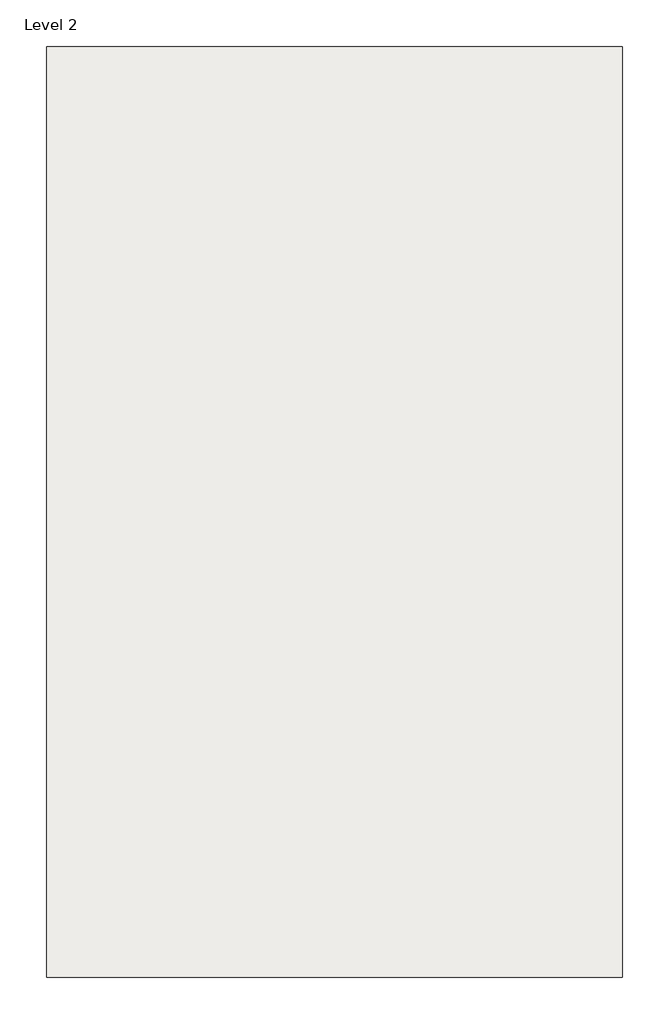
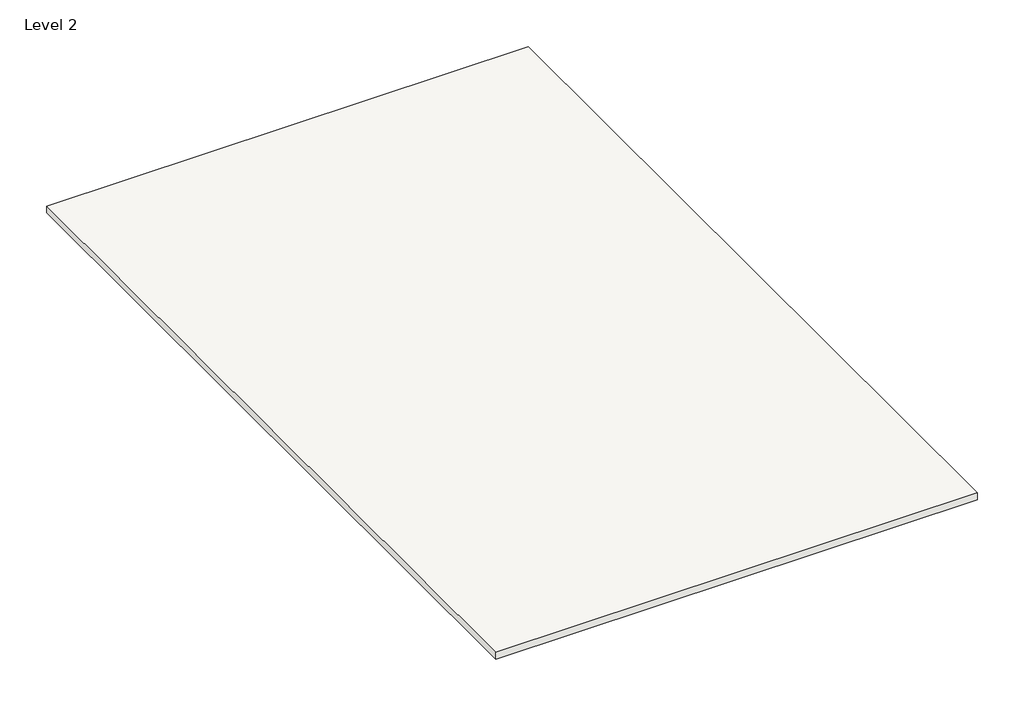
# One storey, incomplete: 1 roof.
"""IFC4 building model written with IfcOpenShell, lengths in millimetres."""

from ifc_helpers import new_model, si_unit, frame, origin, place, context, project, spatial, polyline, outline, extrude, element, save

model = new_model("IFC4")

# Units and contexts
model_context = context("Model", 3, world=origin())
ifc_project = project(units=[si_unit("LENGTHUNIT", "METRE", prefix="MILLI")], contexts=[model_context])

# Site, building, storey
site = spatial("IfcSite", under=ifc_project)
building = spatial("IfcBuilding", under=site)
storey = spatial("IfcBuildingStorey", under=building, Name="Level 2", Elevation=3048.0)

# Roof
placement = place(None, origin())
element("IfcRoof", 1, ObjectType="ROOF 6\"", at=placement, inside=storey, context=model_context, shape_type="SweptSolid", body=[
    extrude(outline(polyline([(-6398.7144966, 6506.3909591), (3888.2855034, 6506.3909591), (3888.2855034, -10115.6142473), (-6398.7144966, -10115.6142473), (-6398.7144966, 6506.3909591)])), frame((0.0, 0.0, 3048.0), z_axis=(0.0, 0.0, 1.0), x_axis=(1.0, 0.0, 0.0)), (0.0, 0.0, 1.0), 152.4),
])

save(model, "model.ifc")

# Revit data of these elements
# Type "ROOF 6\""
#   Assembly Code = "B1020"
#   Layers, outside or top first: 0' - 6" no material (function 1)
# Element 1 (IfcRoof, "ROOF 6\"")
#   built-in parameter 1001705 = 10.5 (stored number, unit not read)
#   built-in parameter 1001710 = 33615
#   Phase Created = New Construction
#   Materials on its faces: "Cherry", "Default Roof", "Softwood, Lumber"
# Materials
#   "Cherry": class "Wood", colour RGB 226 177 128, transparency 0, Description = "Prunus Serotina", Cost = 0
#   "Default Roof": colour RGB 88 101 114, transparency 0, Cost = 0
#   "Softwood, Lumber": class "Wood", colour RGB 223 192 134, transparency 0, Description = "Pinus Echinata", Cost = 0
